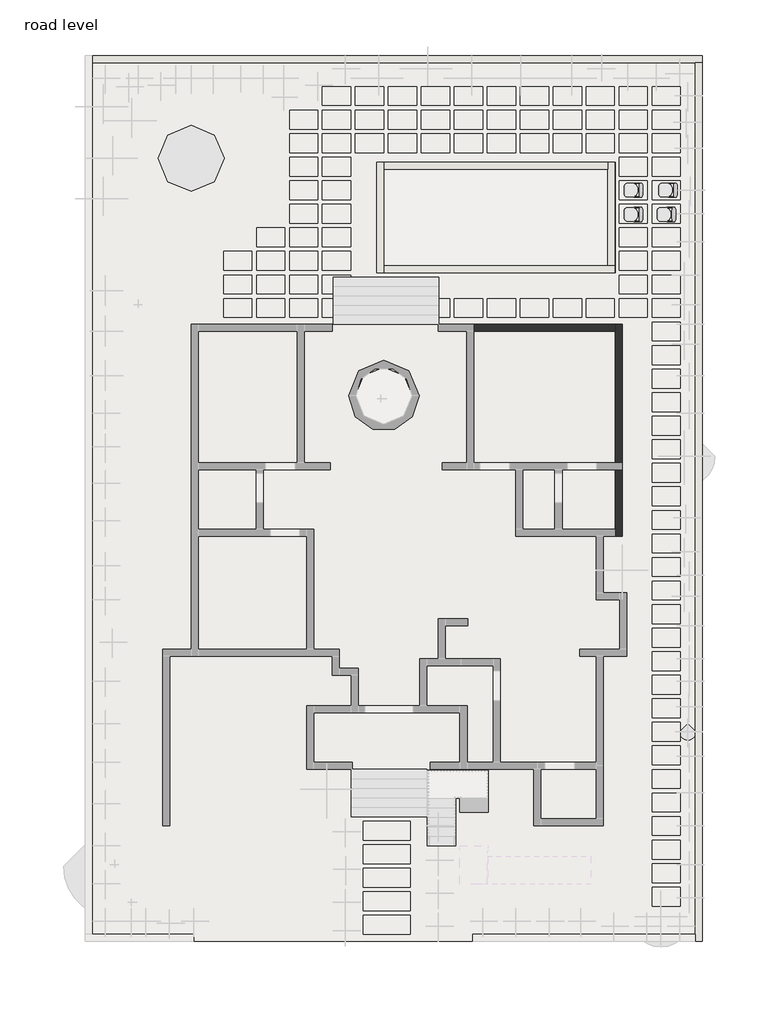
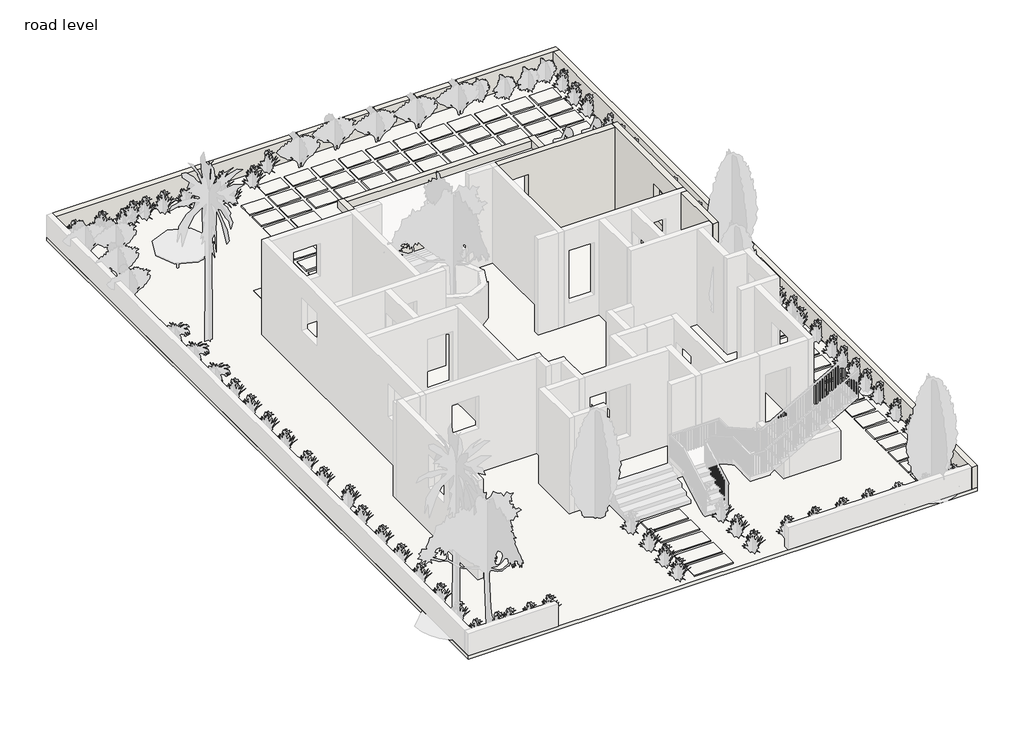
# One storey, part 2 of 5: 9 walls, 2 slabs.
"""IFC4 building model written with IfcOpenShell, lengths in millimetres."""

from ifc_helpers import new_model, si_unit, frame, origin, place, context, project, spatial, polyline, outline, extrude, faceted_brep, element, save

model = new_model("IFC4")

# Units and contexts
model_context = context("Model", 3, world=origin())
ifc_project = project(units=[si_unit("LENGTHUNIT", "METRE", prefix="MILLI")], contexts=[model_context])

# Site, building, storey
site = spatial("IfcSite", under=ifc_project)
building = spatial("IfcBuilding", under=site)
storey = spatial("IfcBuildingStorey", under=building, Name="road level", Elevation=0.0)

# Slabs
placement = place(None, origin())
element("IfcSlab", 1, at=placement, inside=storey, context=model_context, shape_type="SweptSolid", body=[
    extrude(outline(polyline([(3695.0723193, 22227.1086582), (3695.0723193, 21617.5086582), (2780.6723193, 21617.5086582), (2780.6723193, 22227.1086582), (3695.0723193, 22227.1086582)])), frame((0.0, 0.0, -50.8), z_axis=(0.0, 0.0, 1.0), x_axis=(1.0, 0.0, 0.0)), (0.0, 0.0, 1.0), 101.6),
    extrude(outline(polyline([(3695.0723193, 21465.1086582), (3695.0723193, 20855.5086582), (2780.6723193, 20855.5086582), (2780.6723193, 21465.1086582), (3695.0723193, 21465.1086582)])), frame((0.0, 0.0, -50.8), z_axis=(0.0, 0.0, 1.0), x_axis=(1.0, 0.0, 0.0)), (0.0, 0.0, 1.0), 101.6),
    extrude(outline(polyline([(3695.0723193, 20703.1086582), (3695.0723193, 20093.5086582), (2780.6723193, 20093.5086582), (2780.6723193, 20703.1086582), (3695.0723193, 20703.1086582)])), frame((0.0, 0.0, -50.8), z_axis=(0.0, 0.0, 1.0), x_axis=(1.0, 0.0, 0.0)), (0.0, 0.0, 1.0), 101.6),
    extrude(outline(polyline([(3695.0723193, 19941.1086582), (3695.0723193, 19331.5086582), (2780.6723193, 19331.5086582), (2780.6723193, 19941.1086582), (3695.0723193, 19941.1086582)])), frame((0.0, 0.0, -50.8), z_axis=(0.0, 0.0, 1.0), x_axis=(1.0, 0.0, 0.0)), (0.0, 0.0, 1.0), 101.6),
    extrude(outline(polyline([(3695.0723193, 19179.1086582), (3695.0723193, 18569.5086582), (2780.6723193, 18569.5086582), (2780.6723193, 19179.1086582), (3695.0723193, 19179.1086582)])), frame((0.0, 0.0, -50.8), z_axis=(0.0, 0.0, 1.0), x_axis=(1.0, 0.0, 0.0)), (0.0, 0.0, 1.0), 101.6),
    extrude(outline(polyline([(3695.0723193, 18417.1086582), (3695.0723193, 17807.5086582), (2780.6723193, 17807.5086582), (2780.6723193, 18417.1086582), (3695.0723193, 18417.1086582)])), frame((0.0, 0.0, -50.8), z_axis=(0.0, 0.0, 1.0), x_axis=(1.0, 0.0, 0.0)), (0.0, 0.0, 1.0), 101.6),
    extrude(outline(polyline([(3695.0723193, 17655.1086582), (3695.0723193, 17045.5086582), (2780.6723193, 17045.5086582), (2780.6723193, 17655.1086582), (3695.0723193, 17655.1086582)])), frame((0.0, 0.0, -50.8), z_axis=(0.0, 0.0, 1.0), x_axis=(1.0, 0.0, 0.0)), (0.0, 0.0, 1.0), 101.6),
    extrude(outline(polyline([(3695.0723193, 16893.1086582), (3695.0723193, 16283.5086582), (2780.6723193, 16283.5086582), (2780.6723193, 16893.1086582), (3695.0723193, 16893.1086582)])), frame((0.0, 0.0, -50.8), z_axis=(0.0, 0.0, 1.0), x_axis=(1.0, 0.0, 0.0)), (0.0, 0.0, 1.0), 101.6),
    extrude(outline(polyline([(3695.0723193, 16131.1086582), (3695.0723193, 15521.5086582), (2780.6723193, 15521.5086582), (2780.6723193, 16131.1086582), (3695.0723193, 16131.1086582)])), frame((0.0, 0.0, -50.8), z_axis=(0.0, 0.0, 1.0), x_axis=(1.0, 0.0, 0.0)), (0.0, 0.0, 1.0), 101.6),
    extrude(outline(polyline([(3695.0723193, 15369.1086582), (3695.0723193, 14759.5086582), (2780.6723193, 14759.5086582), (2780.6723193, 15369.1086582), (3695.0723193, 15369.1086582)])), frame((0.0, 0.0, -50.8), z_axis=(0.0, 0.0, 1.0), x_axis=(1.0, 0.0, 0.0)), (0.0, 0.0, 1.0), 101.6),
    extrude(outline(polyline([(2628.2723193, 19941.1086582), (2628.2723193, 19331.5086582), (1713.8723193, 19331.5086582), (1713.8723193, 19941.1086582), (2628.2723193, 19941.1086582)])), frame((0.0, 0.0, -50.8), z_axis=(0.0, 0.0, 1.0), x_axis=(1.0, 0.0, 0.0)), (0.0, 0.0, 1.0), 101.6),
    extrude(outline(polyline([(2628.2723193, 19179.1086582), (2628.2723193, 18569.5086582), (1713.8723193, 18569.5086582), (1713.8723193, 19179.1086582), (2628.2723193, 19179.1086582)])), frame((0.0, 0.0, -50.8), z_axis=(0.0, 0.0, 1.0), x_axis=(1.0, 0.0, 0.0)), (0.0, 0.0, 1.0), 101.6),
    extrude(outline(polyline([(2628.2723193, 18417.1086582), (2628.2723193, 17807.5086582), (1713.8723193, 17807.5086582), (1713.8723193, 18417.1086582), (2628.2723193, 18417.1086582)])), frame((0.0, 0.0, -50.8), z_axis=(0.0, 0.0, 1.0), x_axis=(1.0, 0.0, 0.0)), (0.0, 0.0, 1.0), 101.6),
    extrude(outline(polyline([(2628.2723193, 17655.1086582), (2628.2723193, 17045.5086582), (1713.8723193, 17045.5086582), (1713.8723193, 17655.1086582), (2628.2723193, 17655.1086582)])), frame((0.0, 0.0, -50.8), z_axis=(0.0, 0.0, 1.0), x_axis=(1.0, 0.0, 0.0)), (0.0, 0.0, 1.0), 101.6),
    extrude(outline(polyline([(2628.2723193, 16893.1086582), (2628.2723193, 16283.5086582), (1713.8723193, 16283.5086582), (1713.8723193, 16893.1086582), (2628.2723193, 16893.1086582)])), frame((0.0, 0.0, -50.8), z_axis=(0.0, 0.0, 1.0), x_axis=(1.0, 0.0, 0.0)), (0.0, 0.0, 1.0), 101.6),
    extrude(outline(polyline([(2628.2723193, 16131.1086582), (2628.2723193, 15521.5086582), (1713.8723193, 15521.5086582), (1713.8723193, 16131.1086582), (2628.2723193, 16131.1086582)])), frame((0.0, 0.0, -50.8), z_axis=(0.0, 0.0, 1.0), x_axis=(1.0, 0.0, 0.0)), (0.0, 0.0, 1.0), 101.6),
    extrude(outline(polyline([(2628.2723193, 15369.1086582), (2628.2723193, 14759.5086582), (1713.8723193, 14759.5086582), (1713.8723193, 15369.1086582), (2628.2723193, 15369.1086582)])), frame((0.0, 0.0, -50.8), z_axis=(0.0, 0.0, 1.0), x_axis=(1.0, 0.0, 0.0)), (0.0, 0.0, 1.0), 101.6),
    extrude(outline(polyline([(1561.4723193, 17655.1086582), (1561.4723193, 17045.5086582), (647.0723193, 17045.5086582), (647.0723193, 17655.1086582), (1561.4723193, 17655.1086582)])), frame((0.0, 0.0, -50.8), z_axis=(0.0, 0.0, 1.0), x_axis=(1.0, 0.0, 0.0)), (0.0, 0.0, 1.0), 101.6),
    extrude(outline(polyline([(1561.4723193, 16893.1086582), (1561.4723193, 16283.5086582), (647.0723193, 16283.5086582), (647.0723193, 16893.1086582), (1561.4723193, 16893.1086582)])), frame((0.0, 0.0, -50.8), z_axis=(0.0, 0.0, 1.0), x_axis=(1.0, 0.0, 0.0)), (0.0, 0.0, 1.0), 101.6),
    extrude(outline(polyline([(1561.4723193, 16131.1086582), (1561.4723193, 15521.5086582), (647.0723193, 15521.5086582), (647.0723193, 16131.1086582), (1561.4723193, 16131.1086582)])), frame((0.0, 0.0, -50.8), z_axis=(0.0, 0.0, 1.0), x_axis=(1.0, 0.0, 0.0)), (0.0, 0.0, 1.0), 101.6),
    extrude(outline(polyline([(1561.4723193, 15369.1086582), (1561.4723193, 14759.5086582), (647.0723193, 14759.5086582), (647.0723193, 15369.1086582), (1561.4723193, 15369.1086582)])), frame((0.0, 0.0, -50.8), z_axis=(0.0, 0.0, 1.0), x_axis=(1.0, 0.0, 0.0)), (0.0, 0.0, 1.0), 101.6),
    extrude(outline(polyline([(494.6723193, 16893.1086582), (494.6723193, 16283.5086582), (-419.7276807, 16283.5086582), (-419.7276807, 16893.1086582), (494.6723193, 16893.1086582)])), frame((0.0, 0.0, -50.8), z_axis=(0.0, 0.0, 1.0), x_axis=(1.0, 0.0, 0.0)), (0.0, 0.0, 1.0), 101.6),
    extrude(outline(polyline([(494.6723193, 16131.1086582), (494.6723193, 15521.5086582), (-419.7276807, 15521.5086582), (-419.7276807, 16131.1086582), (494.6723193, 16131.1086582)])), frame((0.0, 0.0, -50.8), z_axis=(0.0, 0.0, 1.0), x_axis=(1.0, 0.0, 0.0)), (0.0, 0.0, 1.0), 101.6),
    extrude(outline(polyline([(494.6723193, 15369.1086582), (494.6723193, 14759.5086582), (-419.7276807, 14759.5086582), (-419.7276807, 15369.1086582), (494.6723193, 15369.1086582)])), frame((0.0, 0.0, -50.8), z_axis=(0.0, 0.0, 1.0), x_axis=(1.0, 0.0, 0.0)), (0.0, 0.0, 1.0), 101.6),
    extrude(outline(polyline([(4761.8723193, 22227.1086582), (4761.8723193, 21617.5086582), (3847.4723193, 21617.5086582), (3847.4723193, 22227.1086582), (4761.8723193, 22227.1086582)])), frame((0.0, 0.0, -50.8), z_axis=(0.0, 0.0, 1.0), x_axis=(1.0, 0.0, 0.0)), (0.0, 0.0, 1.0), 101.6),
    extrude(outline(polyline([(4761.8723193, 21465.1086582), (4761.8723193, 20855.5086582), (3847.4723193, 20855.5086582), (3847.4723193, 21465.1086582), (4761.8723193, 21465.1086582)])), frame((0.0, 0.0, -50.8), z_axis=(0.0, 0.0, 1.0), x_axis=(1.0, 0.0, 0.0)), (0.0, 0.0, 1.0), 101.6),
    extrude(outline(polyline([(4761.8723193, 20703.1086582), (4761.8723193, 20093.5086582), (3847.4723193, 20093.5086582), (3847.4723193, 20703.1086582), (4761.8723193, 20703.1086582)])), frame((0.0, 0.0, -50.8), z_axis=(0.0, 0.0, 1.0), x_axis=(1.0, 0.0, 0.0)), (0.0, 0.0, 1.0), 101.6),
    extrude(outline(polyline([(5828.6723193, 22227.1086582), (5828.6723193, 21617.5086582), (4914.2723193, 21617.5086582), (4914.2723193, 22227.1086582), (5828.6723193, 22227.1086582)])), frame((0.0, 0.0, -50.8), z_axis=(0.0, 0.0, 1.0), x_axis=(1.0, 0.0, 0.0)), (0.0, 0.0, 1.0), 101.6),
    extrude(outline(polyline([(5828.6723193, 21465.1086582), (5828.6723193, 20855.5086582), (4914.2723193, 20855.5086582), (4914.2723193, 21465.1086582), (5828.6723193, 21465.1086582)])), frame((0.0, 0.0, -50.8), z_axis=(0.0, 0.0, 1.0), x_axis=(1.0, 0.0, 0.0)), (0.0, 0.0, 1.0), 101.6),
    extrude(outline(polyline([(5828.6723193, 20703.1086582), (5828.6723193, 20093.5086582), (4914.2723193, 20093.5086582), (4914.2723193, 20703.1086582), (5828.6723193, 20703.1086582)])), frame((0.0, 0.0, -50.8), z_axis=(0.0, 0.0, 1.0), x_axis=(1.0, 0.0, 0.0)), (0.0, 0.0, 1.0), 101.6),
    extrude(outline(polyline([(6895.4723193, 22227.1086582), (6895.4723193, 21617.5086582), (5981.0723193, 21617.5086582), (5981.0723193, 22227.1086582), (6895.4723193, 22227.1086582)])), frame((0.0, 0.0, -50.8), z_axis=(0.0, 0.0, 1.0), x_axis=(1.0, 0.0, 0.0)), (0.0, 0.0, 1.0), 101.6),
    extrude(outline(polyline([(6895.4723193, 21465.1086582), (6895.4723193, 20855.5086582), (5981.0723193, 20855.5086582), (5981.0723193, 21465.1086582), (6895.4723193, 21465.1086582)])), frame((0.0, 0.0, -50.8), z_axis=(0.0, 0.0, 1.0), x_axis=(1.0, 0.0, 0.0)), (0.0, 0.0, 1.0), 101.6),
    extrude(outline(polyline([(6895.4723193, 20703.1086582), (6895.4723193, 20093.5086582), (5981.0723193, 20093.5086582), (5981.0723193, 20703.1086582), (6895.4723193, 20703.1086582)])), frame((0.0, 0.0, -50.8), z_axis=(0.0, 0.0, 1.0), x_axis=(1.0, 0.0, 0.0)), (0.0, 0.0, 1.0), 101.6),
    extrude(outline(polyline([(7962.2723193, 22227.1086582), (7962.2723193, 21617.5086582), (7047.8723193, 21617.5086582), (7047.8723193, 22227.1086582), (7962.2723193, 22227.1086582)])), frame((0.0, 0.0, -50.8), z_axis=(0.0, 0.0, 1.0), x_axis=(1.0, 0.0, 0.0)), (0.0, 0.0, 1.0), 101.6),
    extrude(outline(polyline([(7962.2723193, 21465.1086582), (7962.2723193, 20855.5086582), (7047.8723193, 20855.5086582), (7047.8723193, 21465.1086582), (7962.2723193, 21465.1086582)])), frame((0.0, 0.0, -50.8), z_axis=(0.0, 0.0, 1.0), x_axis=(1.0, 0.0, 0.0)), (0.0, 0.0, 1.0), 101.6),
    extrude(outline(polyline([(7962.2723193, 20703.1086582), (7962.2723193, 20093.5086582), (7047.8723193, 20093.5086582), (7047.8723193, 20703.1086582), (7962.2723193, 20703.1086582)])), frame((0.0, 0.0, -50.8), z_axis=(0.0, 0.0, 1.0), x_axis=(1.0, 0.0, 0.0)), (0.0, 0.0, 1.0), 101.6),
    extrude(outline(polyline([(9029.0723193, 22227.1086582), (9029.0723193, 21617.5086582), (8114.6723193, 21617.5086582), (8114.6723193, 22227.1086582), (9029.0723193, 22227.1086582)])), frame((0.0, 0.0, -50.8), z_axis=(0.0, 0.0, 1.0), x_axis=(1.0, 0.0, 0.0)), (0.0, 0.0, 1.0), 101.6),
    extrude(outline(polyline([(9029.0723193, 21465.1086582), (9029.0723193, 20855.5086582), (8114.6723193, 20855.5086582), (8114.6723193, 21465.1086582), (9029.0723193, 21465.1086582)])), frame((0.0, 0.0, -50.8), z_axis=(0.0, 0.0, 1.0), x_axis=(1.0, 0.0, 0.0)), (0.0, 0.0, 1.0), 101.6),
    extrude(outline(polyline([(9029.0723193, 20703.1086582), (9029.0723193, 20093.5086582), (8114.6723193, 20093.5086582), (8114.6723193, 20703.1086582), (9029.0723193, 20703.1086582)])), frame((0.0, 0.0, -50.8), z_axis=(0.0, 0.0, 1.0), x_axis=(1.0, 0.0, 0.0)), (0.0, 0.0, 1.0), 101.6),
    extrude(outline(polyline([(10095.8723193, 22227.1086582), (10095.8723193, 21617.5086582), (9181.4723193, 21617.5086582), (9181.4723193, 22227.1086582), (10095.8723193, 22227.1086582)])), frame((0.0, 0.0, -50.8), z_axis=(0.0, 0.0, 1.0), x_axis=(1.0, 0.0, 0.0)), (0.0, 0.0, 1.0), 101.6),
    extrude(outline(polyline([(10095.8723193, 21465.1086582), (10095.8723193, 20855.5086582), (9181.4723193, 20855.5086582), (9181.4723193, 21465.1086582), (10095.8723193, 21465.1086582)])), frame((0.0, 0.0, -50.8), z_axis=(0.0, 0.0, 1.0), x_axis=(1.0, 0.0, 0.0)), (0.0, 0.0, 1.0), 101.6),
    extrude(outline(polyline([(10095.8723193, 20703.1086582), (10095.8723193, 20093.5086582), (9181.4723193, 20093.5086582), (9181.4723193, 20703.1086582), (10095.8723193, 20703.1086582)])), frame((0.0, 0.0, -50.8), z_axis=(0.0, 0.0, 1.0), x_axis=(1.0, 0.0, 0.0)), (0.0, 0.0, 1.0), 101.6),
    extrude(outline(polyline([(11162.6723193, 22227.1086582), (11162.6723193, 21617.5086582), (10248.2723193, 21617.5086582), (10248.2723193, 22227.1086582), (11162.6723193, 22227.1086582)])), frame((0.0, 0.0, -50.8), z_axis=(0.0, 0.0, 1.0), x_axis=(1.0, 0.0, 0.0)), (0.0, 0.0, 1.0), 101.6),
    extrude(outline(polyline([(11162.6723193, 21465.1086582), (11162.6723193, 20855.5086582), (10248.2723193, 20855.5086582), (10248.2723193, 21465.1086582), (11162.6723193, 21465.1086582)])), frame((0.0, 0.0, -50.8), z_axis=(0.0, 0.0, 1.0), x_axis=(1.0, 0.0, 0.0)), (0.0, 0.0, 1.0), 101.6),
    extrude(outline(polyline([(11162.6723193, 20703.1086582), (11162.6723193, 20093.5086582), (10248.2723193, 20093.5086582), (10248.2723193, 20703.1086582), (11162.6723193, 20703.1086582)])), frame((0.0, 0.0, -50.8), z_axis=(0.0, 0.0, 1.0), x_axis=(1.0, 0.0, 0.0)), (0.0, 0.0, 1.0), 101.6),
    extrude(outline(polyline([(12229.4723193, 22227.1086582), (12229.4723193, 21617.5086582), (11315.0723193, 21617.5086582), (11315.0723193, 22227.1086582), (12229.4723193, 22227.1086582)])), frame((0.0, 0.0, -50.8), z_axis=(0.0, 0.0, 1.0), x_axis=(1.0, 0.0, 0.0)), (0.0, 0.0, 1.0), 101.6),
    extrude(outline(polyline([(12229.4723193, 21465.1086582), (12229.4723193, 20855.5086582), (11315.0723193, 20855.5086582), (11315.0723193, 21465.1086582), (12229.4723193, 21465.1086582)])), frame((0.0, 0.0, -50.8), z_axis=(0.0, 0.0, 1.0), x_axis=(1.0, 0.0, 0.0)), (0.0, 0.0, 1.0), 101.6),
    extrude(outline(polyline([(12229.4723193, 20703.1086582), (12229.4723193, 20093.5086582), (11315.0723193, 20093.5086582), (11315.0723193, 20703.1086582), (12229.4723193, 20703.1086582)])), frame((0.0, 0.0, -50.8), z_axis=(0.0, 0.0, 1.0), x_axis=(1.0, 0.0, 0.0)), (0.0, 0.0, 1.0), 101.6),
    extrude(outline(polyline([(13296.2723193, 22227.1086582), (13296.2723193, 21617.5086582), (12381.8723193, 21617.5086582), (12381.8723193, 22227.1086582), (13296.2723193, 22227.1086582)])), frame((0.0, 0.0, -50.8), z_axis=(0.0, 0.0, 1.0), x_axis=(1.0, 0.0, 0.0)), (0.0, 0.0, 1.0), 101.6),
    extrude(outline(polyline([(13296.2723193, 21465.1086582), (13296.2723193, 20855.5086582), (12381.8723193, 20855.5086582), (12381.8723193, 21465.1086582), (13296.2723193, 21465.1086582)])), frame((0.0, 0.0, -50.8), z_axis=(0.0, 0.0, 1.0), x_axis=(1.0, 0.0, 0.0)), (0.0, 0.0, 1.0), 101.6),
    extrude(outline(polyline([(13296.2723193, 20703.1086582), (13296.2723193, 20093.5086582), (12381.8723193, 20093.5086582), (12381.8723193, 20703.1086582), (13296.2723193, 20703.1086582)])), frame((0.0, 0.0, -50.8), z_axis=(0.0, 0.0, 1.0), x_axis=(1.0, 0.0, 0.0)), (0.0, 0.0, 1.0), 101.6),
    extrude(outline(polyline([(14363.0723193, 22227.1086582), (14363.0723193, 21617.5086582), (13448.6723193, 21617.5086582), (13448.6723193, 22227.1086582), (14363.0723193, 22227.1086582)])), frame((0.0, 0.0, -50.8), z_axis=(0.0, 0.0, 1.0), x_axis=(1.0, 0.0, 0.0)), (0.0, 0.0, 1.0), 101.6),
    extrude(outline(polyline([(14363.0723193, 21465.1086582), (14363.0723193, 20855.5086582), (13448.6723193, 20855.5086582), (13448.6723193, 21465.1086582), (14363.0723193, 21465.1086582)])), frame((0.0, 0.0, -50.8), z_axis=(0.0, 0.0, 1.0), x_axis=(1.0, 0.0, 0.0)), (0.0, 0.0, 1.0), 101.6),
    extrude(outline(polyline([(14363.0723193, 20703.1086582), (14363.0723193, 20093.5086582), (13448.6723193, 20093.5086582), (13448.6723193, 20703.1086582), (14363.0723193, 20703.1086582)])), frame((0.0, 0.0, -50.8), z_axis=(0.0, 0.0, 1.0), x_axis=(1.0, 0.0, 0.0)), (0.0, 0.0, 1.0), 101.6),
    extrude(outline(polyline([(13296.2723193, 19941.1086582), (13296.2723193, 19331.5086582), (12381.8723193, 19331.5086582), (12381.8723193, 19941.1086582), (13296.2723193, 19941.1086582)])), frame((0.0, 0.0, -50.8), z_axis=(0.0, 0.0, 1.0), x_axis=(1.0, 0.0, 0.0)), (0.0, 0.0, 1.0), 101.6),
    extrude(outline(polyline([(14363.0723193, 19941.1086582), (14363.0723193, 19331.5086582), (13448.6723193, 19331.5086582), (13448.6723193, 19941.1086582), (14363.0723193, 19941.1086582)])), frame((0.0, 0.0, -50.8), z_axis=(0.0, 0.0, 1.0), x_axis=(1.0, 0.0, 0.0)), (0.0, 0.0, 1.0), 101.6),
    extrude(outline(polyline([(13296.2723193, 19179.1086582), (13296.2723193, 18569.5086582), (12381.8723193, 18569.5086582), (12381.8723193, 19179.1086582), (13296.2723193, 19179.1086582)])), frame((0.0, 0.0, -50.8), z_axis=(0.0, 0.0, 1.0), x_axis=(1.0, 0.0, 0.0)), (0.0, 0.0, 1.0), 101.6),
    extrude(outline(polyline([(14363.0723193, 19179.1086582), (14363.0723193, 18569.5086582), (13448.6723193, 18569.5086582), (13448.6723193, 19179.1086582), (14363.0723193, 19179.1086582)])), frame((0.0, 0.0, -50.8), z_axis=(0.0, 0.0, 1.0), x_axis=(1.0, 0.0, 0.0)), (0.0, 0.0, 1.0), 101.6),
    extrude(outline(polyline([(13296.2723193, 18417.1086582), (13296.2723193, 17807.5086582), (12381.8723193, 17807.5086582), (12381.8723193, 18417.1086582), (13296.2723193, 18417.1086582)])), frame((0.0, 0.0, -50.8), z_axis=(0.0, 0.0, 1.0), x_axis=(1.0, 0.0, 0.0)), (0.0, 0.0, 1.0), 101.6),
    extrude(outline(polyline([(14363.0723193, 18417.1086582), (14363.0723193, 17807.5086582), (13448.6723193, 17807.5086582), (13448.6723193, 18417.1086582), (14363.0723193, 18417.1086582)])), frame((0.0, 0.0, -50.8), z_axis=(0.0, 0.0, 1.0), x_axis=(1.0, 0.0, 0.0)), (0.0, 0.0, 1.0), 101.6),
    extrude(outline(polyline([(13296.2723193, 17655.1086582), (13296.2723193, 17045.5086582), (12381.8723193, 17045.5086582), (12381.8723193, 17655.1086582), (13296.2723193, 17655.1086582)])), frame((0.0, 0.0, -50.8), z_axis=(0.0, 0.0, 1.0), x_axis=(1.0, 0.0, 0.0)), (0.0, 0.0, 1.0), 101.6),
    extrude(outline(polyline([(14363.0723193, 17655.1086582), (14363.0723193, 17045.5086582), (13448.6723193, 17045.5086582), (13448.6723193, 17655.1086582), (14363.0723193, 17655.1086582)])), frame((0.0, 0.0, -50.8), z_axis=(0.0, 0.0, 1.0), x_axis=(1.0, 0.0, 0.0)), (0.0, 0.0, 1.0), 101.6),
    extrude(outline(polyline([(13296.2723193, 16893.1086582), (13296.2723193, 16283.5086582), (12381.8723193, 16283.5086582), (12381.8723193, 16893.1086582), (13296.2723193, 16893.1086582)])), frame((0.0, 0.0, -50.8), z_axis=(0.0, 0.0, 1.0), x_axis=(1.0, 0.0, 0.0)), (0.0, 0.0, 1.0), 101.6),
    extrude(outline(polyline([(14363.0723193, 16893.1086582), (14363.0723193, 16283.5086582), (13448.6723193, 16283.5086582), (13448.6723193, 16893.1086582), (14363.0723193, 16893.1086582)])), frame((0.0, 0.0, -50.8), z_axis=(0.0, 0.0, 1.0), x_axis=(1.0, 0.0, 0.0)), (0.0, 0.0, 1.0), 101.6),
    extrude(outline(polyline([(13296.2723193, 16131.1086582), (13296.2723193, 15521.5086582), (12381.8723193, 15521.5086582), (12381.8723193, 16131.1086582), (13296.2723193, 16131.1086582)])), frame((0.0, 0.0, -50.8), z_axis=(0.0, 0.0, 1.0), x_axis=(1.0, 0.0, 0.0)), (0.0, 0.0, 1.0), 101.6),
    extrude(outline(polyline([(14363.0723193, 16131.1086582), (14363.0723193, 15521.5086582), (13448.6723193, 15521.5086582), (13448.6723193, 16131.1086582), (14363.0723193, 16131.1086582)])), frame((0.0, 0.0, -50.8), z_axis=(0.0, 0.0, 1.0), x_axis=(1.0, 0.0, 0.0)), (0.0, 0.0, 1.0), 101.6),
    extrude(outline(polyline([(13296.2723193, 15369.1086582), (13296.2723193, 14759.5086582), (12381.8723193, 14759.5086582), (12381.8723193, 15369.1086582), (13296.2723193, 15369.1086582)])), frame((0.0, 0.0, -50.8), z_axis=(0.0, 0.0, 1.0), x_axis=(1.0, 0.0, 0.0)), (0.0, 0.0, 1.0), 101.6),
    extrude(outline(polyline([(14363.0723193, 15369.1086582), (14363.0723193, 14759.5086582), (13448.6723193, 14759.5086582), (13448.6723193, 15369.1086582), (14363.0723193, 15369.1086582)])), frame((0.0, 0.0, -50.8), z_axis=(0.0, 0.0, 1.0), x_axis=(1.0, 0.0, 0.0)), (0.0, 0.0, 1.0), 101.6),
    extrude(outline(polyline([(14363.0723193, 14607.1086582), (14363.0723193, 13997.5086582), (13448.6723193, 13997.5086582), (13448.6723193, 14607.1086582), (14363.0723193, 14607.1086582)])), frame((0.0, 0.0, -50.8), z_axis=(0.0, 0.0, 1.0), x_axis=(1.0, 0.0, 0.0)), (0.0, 0.0, 1.0), 101.6),
    extrude(outline(polyline([(14363.0723193, 13845.1086582), (14363.0723193, 13235.5086582), (13448.6723193, 13235.5086582), (13448.6723193, 13845.1086582), (14363.0723193, 13845.1086582)])), frame((0.0, 0.0, -50.8), z_axis=(0.0, 0.0, 1.0), x_axis=(1.0, 0.0, 0.0)), (0.0, 0.0, 1.0), 101.6),
    extrude(outline(polyline([(14363.0723193, 13083.1086582), (14363.0723193, 12473.5086582), (13448.6723193, 12473.5086582), (13448.6723193, 13083.1086582), (14363.0723193, 13083.1086582)])), frame((0.0, 0.0, -50.8), z_axis=(0.0, 0.0, 1.0), x_axis=(1.0, 0.0, 0.0)), (0.0, 0.0, 1.0), 101.6),
    extrude(outline(polyline([(14363.0723193, 12321.1086582), (14363.0723193, 11711.5086582), (13448.6723193, 11711.5086582), (13448.6723193, 12321.1086582), (14363.0723193, 12321.1086582)])), frame((0.0, 0.0, -50.8), z_axis=(0.0, 0.0, 1.0), x_axis=(1.0, 0.0, 0.0)), (0.0, 0.0, 1.0), 101.6),
    extrude(outline(polyline([(14363.0723193, 11559.1086582), (14363.0723193, 10949.5086582), (13448.6723193, 10949.5086582), (13448.6723193, 11559.1086582), (14363.0723193, 11559.1086582)])), frame((0.0, 0.0, -50.8), z_axis=(0.0, 0.0, 1.0), x_axis=(1.0, 0.0, 0.0)), (0.0, 0.0, 1.0), 101.6),
    extrude(outline(polyline([(14363.0723193, 10797.1086582), (14363.0723193, 10187.5086582), (13448.6723193, 10187.5086582), (13448.6723193, 10797.1086582), (14363.0723193, 10797.1086582)])), frame((0.0, 0.0, -50.8), z_axis=(0.0, 0.0, 1.0), x_axis=(1.0, 0.0, 0.0)), (0.0, 0.0, 1.0), 101.6),
    extrude(outline(polyline([(14363.0723193, 10035.1086582), (14363.0723193, 9425.5086582), (13448.6723193, 9425.5086582), (13448.6723193, 10035.1086582), (14363.0723193, 10035.1086582)])), frame((0.0, 0.0, -50.8), z_axis=(0.0, 0.0, 1.0), x_axis=(1.0, 0.0, 0.0)), (0.0, 0.0, 1.0), 101.6),
    extrude(outline(polyline([(14363.0723193, 9273.1086582), (14363.0723193, 8663.5086582), (13448.6723193, 8663.5086582), (13448.6723193, 9273.1086582), (14363.0723193, 9273.1086582)])), frame((0.0, 0.0, -50.8), z_axis=(0.0, 0.0, 1.0), x_axis=(1.0, 0.0, 0.0)), (0.0, 0.0, 1.0), 101.6),
    extrude(outline(polyline([(14363.0723193, 8511.1086582), (14363.0723193, 7901.5086582), (13448.6723193, 7901.5086582), (13448.6723193, 8511.1086582), (14363.0723193, 8511.1086582)])), frame((0.0, 0.0, -50.8), z_axis=(0.0, 0.0, 1.0), x_axis=(1.0, 0.0, 0.0)), (0.0, 0.0, 1.0), 101.6),
    extrude(outline(polyline([(14363.0723193, 7749.1086582), (14363.0723193, 7139.5086582), (13448.6723193, 7139.5086582), (13448.6723193, 7749.1086582), (14363.0723193, 7749.1086582)])), frame((0.0, 0.0, -50.8), z_axis=(0.0, 0.0, 1.0), x_axis=(1.0, 0.0, 0.0)), (0.0, 0.0, 1.0), 101.6),
    extrude(outline(polyline([(14363.0723193, 6987.1086582), (14363.0723193, 6377.5086582), (13448.6723193, 6377.5086582), (13448.6723193, 6987.1086582), (14363.0723193, 6987.1086582)])), frame((0.0, 0.0, -50.8), z_axis=(0.0, 0.0, 1.0), x_axis=(1.0, 0.0, 0.0)), (0.0, 0.0, 1.0), 101.6),
    extrude(outline(polyline([(14363.0723193, 6225.1086582), (14363.0723193, 5615.5086582), (13448.6723193, 5615.5086582), (13448.6723193, 6225.1086582), (14363.0723193, 6225.1086582)])), frame((0.0, 0.0, -50.8), z_axis=(0.0, 0.0, 1.0), x_axis=(1.0, 0.0, 0.0)), (0.0, 0.0, 1.0), 101.6),
    extrude(outline(polyline([(14363.0723193, 5463.1086582), (14363.0723193, 4853.5086582), (13448.6723193, 4853.5086582), (13448.6723193, 5463.1086582), (14363.0723193, 5463.1086582)])), frame((0.0, 0.0, -50.8), z_axis=(0.0, 0.0, 1.0), x_axis=(1.0, 0.0, 0.0)), (0.0, 0.0, 1.0), 101.6),
    extrude(outline(polyline([(14363.0723193, 4701.1086582), (14363.0723193, 4091.5086582), (13448.6723193, 4091.5086582), (13448.6723193, 4701.1086582), (14363.0723193, 4701.1086582)])), frame((0.0, 0.0, -50.8), z_axis=(0.0, 0.0, 1.0), x_axis=(1.0, 0.0, 0.0)), (0.0, 0.0, 1.0), 101.6),
    extrude(outline(polyline([(14363.0723193, 3939.1086582), (14363.0723193, 3329.5086582), (13448.6723193, 3329.5086582), (13448.6723193, 3939.1086582), (14363.0723193, 3939.1086582)])), frame((0.0, 0.0, -50.8), z_axis=(0.0, 0.0, 1.0), x_axis=(1.0, 0.0, 0.0)), (0.0, 0.0, 1.0), 101.6),
    extrude(outline(polyline([(14363.0723193, 3177.1086582), (14363.0723193, 2567.5086582), (13448.6723193, 2567.5086582), (13448.6723193, 3177.1086582), (14363.0723193, 3177.1086582)])), frame((0.0, 0.0, -50.8), z_axis=(0.0, 0.0, 1.0), x_axis=(1.0, 0.0, 0.0)), (0.0, 0.0, 1.0), 101.6),
    extrude(outline(polyline([(14363.0723193, 2415.1086582), (14363.0723193, 1805.5086582), (13448.6723193, 1805.5086582), (13448.6723193, 2415.1086582), (14363.0723193, 2415.1086582)])), frame((0.0, 0.0, -50.8), z_axis=(0.0, 0.0, 1.0), x_axis=(1.0, 0.0, 0.0)), (0.0, 0.0, 1.0), 101.6),
    extrude(outline(polyline([(14363.0723193, 1653.1086582), (14363.0723193, 1043.5086582), (13448.6723193, 1043.5086582), (13448.6723193, 1653.1086582), (14363.0723193, 1653.1086582)])), frame((0.0, 0.0, -50.8), z_axis=(0.0, 0.0, 1.0), x_axis=(1.0, 0.0, 0.0)), (0.0, 0.0, 1.0), 101.6),
    extrude(outline(polyline([(14363.0723193, 891.1086582), (14363.0723193, 281.5086582), (13448.6723193, 281.5086582), (13448.6723193, 891.1086582), (14363.0723193, 891.1086582)])), frame((0.0, 0.0, -50.8), z_axis=(0.0, 0.0, 1.0), x_axis=(1.0, 0.0, 0.0)), (0.0, 0.0, 1.0), 101.6),
    extrude(outline(polyline([(14363.0723193, 129.1086582), (14363.0723193, -480.4913418), (13448.6723193, -480.4913418), (13448.6723193, 129.1086582), (14363.0723193, 129.1086582)])), frame((0.0, 0.0, -50.8), z_axis=(0.0, 0.0, 1.0), x_axis=(1.0, 0.0, 0.0)), (0.0, 0.0, 1.0), 101.6),
    extrude(outline(polyline([(14363.0723193, -632.8913418), (14363.0723193, -1242.4913418), (13448.6723193, -1242.4913418), (13448.6723193, -632.8913418), (14363.0723193, -632.8913418)])), frame((0.0, 0.0, -50.8), z_axis=(0.0, 0.0, 1.0), x_axis=(1.0, 0.0, 0.0)), (0.0, 0.0, 1.0), 101.6),
    extrude(outline(polyline([(14363.0723193, -1394.8913418), (14363.0723193, -2004.4913418), (13448.6723193, -2004.4913418), (13448.6723193, -1394.8913418), (14363.0723193, -1394.8913418)])), frame((0.0, 0.0, -50.8), z_axis=(0.0, 0.0, 1.0), x_axis=(1.0, 0.0, 0.0)), (0.0, 0.0, 1.0), 101.6),
    extrude(outline(polyline([(14363.0723193, -2156.8913418), (14363.0723193, -2766.4913418), (13448.6723193, -2766.4913418), (13448.6723193, -2156.8913418), (14363.0723193, -2156.8913418)])), frame((0.0, 0.0, -50.8), z_axis=(0.0, 0.0, 1.0), x_axis=(1.0, 0.0, 0.0)), (0.0, 0.0, 1.0), 101.6),
    extrude(outline(polyline([(14363.0723193, -2918.8913418), (14363.0723193, -3528.4913418), (13448.6723193, -3528.4913418), (13448.6723193, -2918.8913418), (14363.0723193, -2918.8913418)])), frame((0.0, 0.0, -50.8), z_axis=(0.0, 0.0, 1.0), x_axis=(1.0, 0.0, 0.0)), (0.0, 0.0, 1.0), 101.6),
    extrude(outline(polyline([(14363.0723193, -3680.8913418), (14363.0723193, -4290.4913418), (13448.6723193, -4290.4913418), (13448.6723193, -3680.8913418), (14363.0723193, -3680.8913418)])), frame((0.0, 0.0, -50.8), z_axis=(0.0, 0.0, 1.0), x_axis=(1.0, 0.0, 0.0)), (0.0, 0.0, 1.0), 101.6),
    extrude(outline(polyline([(5624.4340664, -1542.8713978), (5624.4340664, -2152.4713978), (4100.4340664, -2152.4713978), (4100.4340664, -1542.8713978), (5624.4340664, -1542.8713978)])), frame((0.0, 0.0, -50.8), z_axis=(0.0, 0.0, 1.0), x_axis=(1.0, 0.0, 0.0)), (0.0, 0.0, 1.0), 101.6),
    extrude(outline(polyline([(5624.4340664, -2304.8713978), (5624.4340664, -2914.4713978), (4100.4340664, -2914.4713978), (4100.4340664, -2304.8713978), (5624.4340664, -2304.8713978)])), frame((0.0, 0.0, -50.8), z_axis=(0.0, 0.0, 1.0), x_axis=(1.0, 0.0, 0.0)), (0.0, 0.0, 1.0), 101.6),
    extrude(outline(polyline([(5624.4340664, -3066.8713978), (5624.4340664, -3676.4713978), (4100.4340664, -3676.4713978), (4100.4340664, -3066.8713978), (5624.4340664, -3066.8713978)])), frame((0.0, 0.0, -50.8), z_axis=(0.0, 0.0, 1.0), x_axis=(1.0, 0.0, 0.0)), (0.0, 0.0, 1.0), 101.6),
    extrude(outline(polyline([(5624.4340664, -3828.8713978), (5624.4340664, -4438.4713978), (4100.4340664, -4438.4713978), (4100.4340664, -3828.8713978), (5624.4340664, -3828.8713978)])), frame((0.0, 0.0, -50.8), z_axis=(0.0, 0.0, 1.0), x_axis=(1.0, 0.0, 0.0)), (0.0, 0.0, 1.0), 101.6),
    extrude(outline(polyline([(5624.4340664, -4590.8713978), (5624.4340664, -5200.4713978), (4100.4340664, -5200.4713978), (4100.4340664, -4590.8713978), (5624.4340664, -4590.8713978)])), frame((0.0, 0.0, -50.8), z_axis=(0.0, 0.0, 1.0), x_axis=(1.0, 0.0, 0.0)), (0.0, 0.0, 1.0), 101.6),
    extrude(outline(polyline([(4761.8723193, 15369.1086582), (4761.8723193, 14759.5086582), (3847.4723193, 14759.5086582), (3847.4723193, 15369.1086582), (4761.8723193, 15369.1086582)])), frame((0.0, 0.0, -50.8), z_axis=(0.0, 0.0, 1.0), x_axis=(1.0, 0.0, 0.0)), (0.0, 0.0, 1.0), 101.6),
    extrude(outline(polyline([(5828.6723193, 15369.1086582), (5828.6723193, 14759.5086582), (4914.2723193, 14759.5086582), (4914.2723193, 15369.1086582), (5828.6723193, 15369.1086582)])), frame((0.0, 0.0, -50.8), z_axis=(0.0, 0.0, 1.0), x_axis=(1.0, 0.0, 0.0)), (0.0, 0.0, 1.0), 101.6),
    extrude(outline(polyline([(6895.4723193, 15369.1086582), (6895.4723193, 14759.5086582), (5981.0723193, 14759.5086582), (5981.0723193, 15369.1086582), (6895.4723193, 15369.1086582)])), frame((0.0, 0.0, -50.8), z_axis=(0.0, 0.0, 1.0), x_axis=(1.0, 0.0, 0.0)), (0.0, 0.0, 1.0), 101.6),
    extrude(outline(polyline([(7962.2723193, 15369.1086582), (7962.2723193, 14759.5086582), (7047.8723193, 14759.5086582), (7047.8723193, 15369.1086582), (7962.2723193, 15369.1086582)])), frame((0.0, 0.0, -50.8), z_axis=(0.0, 0.0, 1.0), x_axis=(1.0, 0.0, 0.0)), (0.0, 0.0, 1.0), 101.6),
    extrude(outline(polyline([(9029.0723193, 15369.1086582), (9029.0723193, 14759.5086582), (8114.6723193, 14759.5086582), (8114.6723193, 15369.1086582), (9029.0723193, 15369.1086582)])), frame((0.0, 0.0, -50.8), z_axis=(0.0, 0.0, 1.0), x_axis=(1.0, 0.0, 0.0)), (0.0, 0.0, 1.0), 101.6),
    extrude(outline(polyline([(10095.8723193, 15369.1086582), (10095.8723193, 14759.5086582), (9181.4723193, 14759.5086582), (9181.4723193, 15369.1086582), (10095.8723193, 15369.1086582)])), frame((0.0, 0.0, -50.8), z_axis=(0.0, 0.0, 1.0), x_axis=(1.0, 0.0, 0.0)), (0.0, 0.0, 1.0), 101.6),
    extrude(outline(polyline([(11162.6723193, 15369.1086582), (11162.6723193, 14759.5086582), (10248.2723193, 14759.5086582), (10248.2723193, 15369.1086582), (11162.6723193, 15369.1086582)])), frame((0.0, 0.0, -50.8), z_axis=(0.0, 0.0, 1.0), x_axis=(1.0, 0.0, 0.0)), (0.0, 0.0, 1.0), 101.6),
    extrude(outline(polyline([(12229.4723193, 15369.1086582), (12229.4723193, 14759.5086582), (11315.0723193, 14759.5086582), (11315.0723193, 15369.1086582), (12229.4723193, 15369.1086582)])), frame((0.0, 0.0, -50.8), z_axis=(0.0, 0.0, 1.0), x_axis=(1.0, 0.0, 0.0)), (0.0, 0.0, 1.0), 101.6),
    extrude(outline(polyline([(2628.2723193, 20703.1086582), (2628.2723193, 20093.5086582), (1713.8723193, 20093.5086582), (1713.8723193, 20703.1086582), (2628.2723193, 20703.1086582)])), frame((0.0, 0.0, -50.8), z_axis=(0.0, 0.0, 1.0), x_axis=(1.0, 0.0, 0.0)), (0.0, 0.0, 1.0), 101.6),
    extrude(outline(polyline([(2628.2723193, 21465.1086582), (2628.2723193, 20855.5086582), (1713.8723193, 20855.5086582), (1713.8723193, 21465.1086582), (2628.2723193, 21465.1086582)])), frame((0.0, 0.0, -50.8), z_axis=(0.0, 0.0, 1.0), x_axis=(1.0, 0.0, 0.0)), (0.0, 0.0, 1.0), 101.6),
])
element("IfcSlab", 2, at=placement, inside=storey, context=model_context, shape_type="SweptSolid", body=[
    extrude(outline(polyline([(15065.8512825, 23221.0906886), (15065.8512825, -5430.1093114), (-4898.5487175, -5430.1093114), (-4898.5487175, 23221.0906886), (15065.8512825, 23221.0906886)]), holes=[polyline([(12246.4512825, 16197.9906886), (12246.4512825, 19779.3906886), (4540.3394971, 19779.3906886), (4540.3394971, 16197.9906886), (12246.4512825, 16197.9906886)])]), frame((0.0, 0.0, -152.4), z_axis=(0.0, 0.0, 1.0), x_axis=(1.0, 0.0, 0.0)), (0.0, 0.0, 1.0), 152.4),
])

# Walls
element("IfcWall", 3, at=placement, inside=storey, context=model_context, shape_type="Brep", body=[
    faceted_brep([(12475.0512825, 10063.8906886, 0.0), (12475.0512825, 14534.2906886, 0.0), (12475.0512825, 14534.2906886, 3962.4), (12475.0512825, 10063.8906886, 3962.4), (12475.0512825, 10648.0906886, 3175.0), (12475.0512825, 11689.4906886, 3175.0), (12475.0512825, 11689.4906886, 1828.8), (12475.0512825, 10648.0906886, 1828.8), (12246.4512825, 10063.8906886, 0.0), (12246.4512825, 10063.8906886, 3962.4), (12246.4512825, 14305.6906886, 3962.4), (12246.4512825, 14534.2906886, 3962.4), (12246.4512825, 14534.2906886, 0.0), (12246.4512825, 14305.6906886, 0.0), (12246.4512825, 10648.0906886, 3175.0), (12246.4512825, 10648.0906886, 1828.8), (12246.4512825, 11689.4906886, 1828.8), (12246.4512825, 11689.4906886, 3175.0)], [[[0, 1, 2, 3], [4, 5, 6, 7]], [[8, 9, 10, 11, 12, 13], [14, 15, 16, 17]], [[1, 0, 8, 13, 12]], [[0, 3, 9, 8]], [[2, 1, 12, 11]], [[3, 2, 11, 10, 9]], [[15, 14, 4, 7]], [[16, 15, 7, 6]], [[17, 16, 6, 5]], [[14, 17, 5, 4]]]),
])
element("IfcWall", 4, at=placement, inside=storey, context=model_context, shape_type="SweptSolid", body=[
    extrude(outline(polyline([(0.0, 12246.4512825), (3962.4, 12246.4512825), (3962.4, 7674.4512825), (0.0, 7674.4512825), (0.0, 12246.4512825)]), holes=[polyline([(3175.0, 8842.8512825), (1828.8, 8842.8512825), (1828.8, 7801.4512825), (3175.0, 7801.4512825), (3175.0, 8842.8512825)])]), frame((0.0, 14305.6906886, 0.0), z_axis=(0.0, 1.0, 0.0), x_axis=(0.0, 0.0, 1.0)), (0.0, 0.0, 1.0), 228.6),
])
element("IfcWall", 5, at=placement, inside=storey, context=model_context, shape_type="Brep", body=[
    faceted_brep([(12246.4512825, 9835.2906886, 0.0), (12246.4512825, 7904.8906886, 0.0), (12246.4512825, 7676.2906886, 0.0), (12246.4512825, 7676.2906886, 3962.4), (12246.4512825, 7904.8906886, 3962.4), (12246.4512825, 9835.2906886, 3962.4), (12475.0512825, 9835.2906886, 0.0), (12475.0512825, 9835.2906886, 3962.4), (12475.0512825, 7676.2906886, 3962.4), (12475.0512825, 7676.2906886, 0.0)], [[[0, 1, 2, 3, 4, 5]], [[6, 7, 8, 9]], [[2, 1, 0, 6, 9]], [[0, 5, 7, 6]], [[3, 2, 9, 8]], [[5, 4, 3, 8, 7]]]),
])
element("IfcWall", 6, at=placement, inside=storey, context=model_context, shape_type="Brep", body=[
    faceted_brep([(4540.3394971, 19779.3906886, -1828.8), (4540.3394971, 16197.9906886, -1828.8), (4540.3394971, 16197.9906886, 304.8), (4540.3394971, 19779.3906886, 304.8), (4768.9394971, 19779.3906886, -1828.8), (4768.9394971, 19779.3906886, 304.8), (4768.9394971, 19550.7906886, 304.8), (4768.9394971, 16426.5906886, 304.8), (4768.9394971, 16197.9906886, 304.8), (4768.9394971, 16197.9906886, -1828.8), (4768.9394971, 16426.5906886, -1828.8), (4768.9394971, 19550.7906886, -1828.8)], [[[0, 1, 2, 3]], [[4, 5, 6, 7, 8, 9, 10, 11]], [[1, 0, 4, 11, 10, 9]], [[3, 2, 8, 7, 6, 5]], [[2, 1, 9, 8]], [[0, 3, 5, 4]]]),
])
element("IfcWall", 7, at=placement, inside=storey, context=model_context, shape_type="Brep", body=[
    faceted_brep([(4768.9394971, 16197.9906886, -1828.8), (12236.5394971, 16197.9906886, -1828.8), (12236.5394971, 16197.9906886, 304.8), (4768.9394971, 16197.9906886, 304.8), (4768.9394971, 16426.5906886, -1828.8), (4768.9394971, 16426.5906886, 304.8), (12007.9394971, 16426.5906886, 304.8), (12236.5394971, 16426.5906886, 304.8), (12236.5394971, 16426.5906886, -1828.8), (12007.9394971, 16426.5906886, -1828.8)], [[[0, 1, 2, 3]], [[4, 5, 6, 7, 8, 9]], [[1, 0, 4, 9, 8]], [[3, 2, 7, 6, 5]], [[0, 3, 5, 4]], [[2, 1, 8, 7]]]),
])
element("IfcWall", 8, at=placement, inside=storey, context=model_context, shape_type="Brep", body=[
    faceted_brep([(12236.5394971, 16426.5906886, -1828.8), (12236.5394971, 19779.3906886, -1828.8), (12236.5394971, 19779.3906886, 304.8), (12236.5394971, 16426.5906886, 304.8), (12007.9394971, 16426.5906886, -1828.8), (12007.9394971, 16426.5906886, 304.8), (12007.9394971, 19550.7906886, 304.8), (12007.9394971, 19779.3906886, 304.8), (12007.9394971, 19779.3906886, -1828.8), (12007.9394971, 19550.7906886, -1828.8)], [[[0, 1, 2, 3]], [[4, 5, 6, 7, 8, 9]], [[1, 0, 4, 9, 8]], [[3, 2, 7, 6, 5]], [[0, 3, 5, 4]], [[2, 1, 8, 7]]]),
])
element("IfcWall", 9, at=placement, inside=storey, context=model_context, shape_type="Brep", body=[
    faceted_brep([(-4669.9487175, 22992.4906886, 0.0), (14837.2512825, 22992.4906886, 0.0), (15065.8512825, 22992.4906886, 0.0), (15065.8512825, 22992.4906886, 914.4), (14837.2512825, 22992.4906886, 914.4), (-4669.9487175, 22992.4906886, 914.4), (-4669.9487175, 23221.0906886, 0.0), (-4669.9487175, 23221.0906886, 914.4), (15065.8512825, 23221.0906886, 914.4), (15065.8512825, 23221.0906886, 0.0)], [[[0, 1, 2, 3, 4, 5]], [[6, 7, 8, 9]], [[2, 1, 0, 6, 9]], [[5, 4, 3, 8, 7]], [[3, 2, 9, 8]], [[0, 5, 7, 6]]]),
])
element("IfcWall", 10, at=placement, inside=storey, context=model_context, shape_type="Brep", body=[
    faceted_brep([(14837.2512825, 22992.4906886, 0.0), (14837.2512825, -5201.5093114, 0.0), (14837.2512825, -5430.1093114, 0.0), (14837.2512825, -5430.1093114, 914.4), (14837.2512825, -5201.5093114, 914.4), (14837.2512825, 22992.4906886, 914.4), (15065.8512825, 22992.4906886, 0.0), (15065.8512825, 22992.4906886, 914.4), (15065.8512825, -5430.1093114, 914.4), (15065.8512825, -5430.1093114, 0.0)], [[[0, 1, 2, 3, 4, 5]], [[6, 7, 8, 9]], [[2, 1, 0, 6, 9]], [[5, 4, 3, 8, 7]], [[0, 5, 7, 6]], [[3, 2, 9, 8]]]),
])
element("IfcWall", 11, at=placement, inside=storey, context=model_context, shape_type="SweptSolid", body=[
    extrude(outline(polyline([(12007.9394971, 19550.7906886), (4768.9394971, 19550.7906886), (4768.9394971, 19779.3906886), (12007.9394971, 19779.3906886), (12007.9394971, 19550.7906886)])), frame((0.0, 0.0, -1828.8), z_axis=(0.0, 0.0, 1.0), x_axis=(1.0, 0.0, 0.0)), (0.0, 0.0, 1.0), 2133.6),
])

save(model, "model.ifc")

# Revit data of these elements
# Type
#   Assembly Code = "B1010"
#   Function = 0
#   Layers, outside or top first: 0' - 4" "Concrete, Cast-in-Place gray" (function 1)
# Type
#   Assembly Code = "B1010"
#   Function = 0
#   Layers, outside or top first: 0' - 6" "Grass" (function 1)
# Type
#   Assembly Code = "B2010"
#   Layers, outside or top first: 0' - 9" no material (function 1)
# Element 1 (IfcSlab)
#   Height Offset From Level = 0' - 2"
#   Phase Created = New Construction
#   Materials on its faces: "Concrete, Cast-in-Place gray"
# Element 2 (IfcSlab)
#   Height Offset From Level = 0' - 0"
#   Phase Created = New Construction
#   Materials on its faces: "Grass"
# Elements 3, 4, 5 (IfcWall)
#   Top Offset = 0' - 0"
#   Base Offset = 0' - 0"
#   wall height = 13' - 0"
#   Phase Created = New Construction
#   Base Constraint = road level
#   Top Constraint = 1ST FLOOR
#   Materials on its faces: "Default Wall"
# Elements 6, 7, 8, 11 (IfcWall)
#   built-in parameter 1001111 = -6' - 0"
#   Top Offset = 0' - 0"
#   Base Offset = -6' - 0"
#   Unconnected Height = 7' - 0"
#   wall height = 7' - 0"
#   Phase Created = New Construction
#   Base Constraint = road level
#   Materials on its faces: "Default Wall"
# Elements 9, 10 (IfcWall)
#   Top Offset = 0' - 0"
#   Base Offset = 0' - 0"
#   wall height = 3' - 0"
#   Phase Created = New Construction
#   Base Constraint = road level
#   Top Constraint = GF FLOOR
#   Materials on its faces: "Default Wall"
# Materials
#   "Concrete, Cast-in-Place gray": class "Concrete", colour RGB 192 192 192, transparency 0, Description = "Cast-in-place concrete", Cost = 0
#   "Grass": class "Generic", colour RGB 104 137 66, transparency 0, Description = "Physical material.", Cost = 0
#   "Default Wall": colour RGB 128 128 128, transparency 0, Cost = 0
